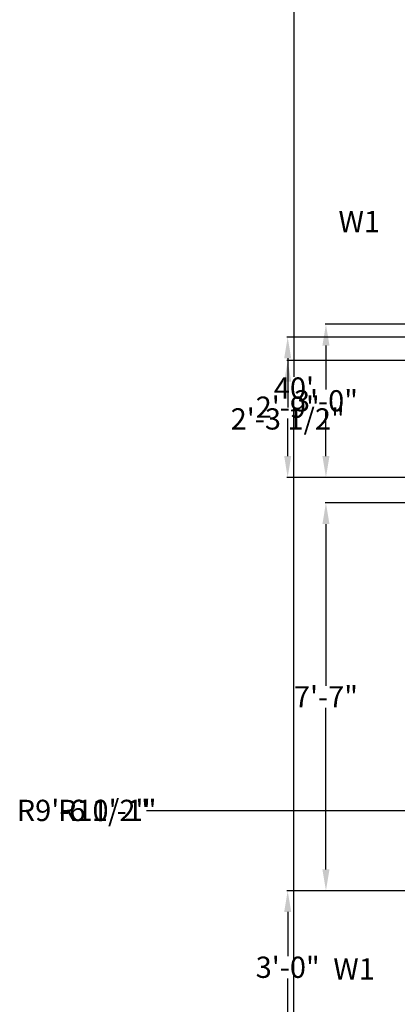
# Model space of a CAD drawing. Units: inches. Extents: x 3136 to 3620, y 13606 to 14152.
# Tile 2 of 6: x 3136 to 3225, y 13734 to 13965. Entities that reach past the tile are written whole.
import ezdxf

# ---------------------------------------------------------------- set-up
doc = ezdxf.new("R2010")
doc.units = ezdxf.units.IN
doc.layers.add('A-ANNO-DIMS', color=2, linetype='Continuous', lineweight=18)
doc.layers.add('A-ANNO-TEXT', color=7, linetype='Continuous', lineweight=18)
doc.styles.get("Standard").update_dxf_attribs({"font": 'arial.ttf', "height": 5})
doc.dimstyles.get("Standard").update_dxf_attribs({"dimtxt": 5, "dimasz": 5, "dimexe": 0.18, "dimexo": 0.0625, "dimgap": 0.09, "dimtad": 0, "dimtih": 1, "dimtoh": 1, "dimdec": 0, "dimzin": 0, "dimdsep": 46, "dimlunit": 3, "dimtxsty": 'Standard', "dimcen": 0.09, "dimadec": 0, "dimazin": 0, "dimtfac": 1, "dimtdec": 0, "dimtofl": 0, "dimtmove": 0, "dimatfit": 3, "dimfxl": 1, "dimtolj": 1, "dimtzin": 0, "dimarcsym": 0})

# ---------------------------------------------------------------- blocks, each defined once
blk = doc.blocks.new('*D28')
at = {"layer": 'A-ANNO-DIMS', "color": 0, "lineweight": -2, "transparency": 16777216}
for p, q in [((3224.81, 14118.84), (3200.37, 14118.84)), ((3200.55, 14113.84), (3200.55, 13881.48)), ((3200.55, 13643.84), (3200.55, 13876.2)), ((3224.81, 13638.84), (3200.37, 13638.84))]:
    blk.add_line(p, q, dxfattribs=at)
at = {"layer": 'A-ANNO-DIMS', "color": 0, "transparency": 16777216}
for points in [[(3199.71, 14113.84), (3201.38, 14113.84), (3200.55, 14118.84)], [(3199.71, 13643.84), (3201.38, 13643.84), (3200.55, 13638.84)]]:
    blk.add_solid(points, dxfattribs=at)
at = {"layer": 'Defpoints', "color": 0, "transparency": 16777216}
for p in [(3200.55, 14118.84), (3224.87, 14118.84), (3224.87, 13638.84)]:
    blk.add_point(p, dxfattribs=at)
at = {"layer": 'A-ANNO-DIMS', "color": 0, "transparency": 16777216, "insert": (3200.55, 13878.84), "char_height": 5, "attachment_point": 5}
blk.add_mtext("\\A1;40'", dxfattribs=at)
blk = doc.blocks.new('*D49')
at = {"layer": 'A-ANNO-DIMS', "color": 0, "lineweight": -2, "transparency": 16777216}
for p, q in [((3503.81, 13885.32), (3198.89, 13885.32)), ((3199.07, 13880.32), (3199.07, 13874.26)), ((3199.07, 13862.84), (3199.07, 13868.9)), ((3503.81, 13857.84), (3198.89, 13857.84))]:
    blk.add_line(p, q, dxfattribs=at)
at = {"layer": 'A-ANNO-DIMS', "color": 0, "transparency": 16777216}
for points in [[(3198.24, 13880.32), (3199.9, 13880.32), (3199.07, 13885.32)], [(3198.24, 13862.84), (3199.9, 13862.84), (3199.07, 13857.84)]]:
    blk.add_solid(points, dxfattribs=at)
at = {"layer": 'Defpoints', "color": 0, "transparency": 16777216}
for p in [(3199.07, 13885.32), (3503.87, 13885.32), (3503.87, 13857.84)]:
    blk.add_point(p, dxfattribs=at)
at = {"layer": 'A-ANNO-DIMS', "color": 0, "transparency": 16777216, "insert": (3199.07, 13871.58), "char_height": 5, "attachment_point": 5}
blk.add_mtext('\\A1;2\'-3 1/2"', dxfattribs=at)
blk = doc.blocks.new('*D51')
at = {"layer": 'A-ANNO-DIMS', "color": 0, "lineweight": -2, "transparency": 16777216}
for p, q in [((3224.81, 13760.63), (3198.89, 13760.63)), ((3199.07, 13755.63), (3199.07, 13745.27)), ((3199.07, 13729.63), (3199.07, 13739.99)), ((3224.81, 13724.63), (3198.89, 13724.63))]:
    blk.add_line(p, q, dxfattribs=at)
at = {"layer": 'A-ANNO-DIMS', "color": 0, "transparency": 16777216}
for points in [[(3198.24, 13755.63), (3199.9, 13755.63), (3199.07, 13760.63)], [(3198.24, 13729.63), (3199.9, 13729.63), (3199.07, 13724.63)]]:
    blk.add_solid(points, dxfattribs=at)
at = {"layer": 'Defpoints', "color": 0, "transparency": 16777216}
for p in [(3199.07, 13760.63), (3224.87, 13760.63), (3224.87, 13724.63)]:
    blk.add_point(p, dxfattribs=at)
at = {"layer": 'A-ANNO-DIMS', "color": 0, "transparency": 16777216, "insert": (3199.07, 13742.63), "char_height": 5, "attachment_point": 5}
blk.add_mtext('\\A1;3\'-0"', dxfattribs=at)
blk = doc.blocks.new('*D63')
at = {"layer": 'A-ANNO-DIMS', "color": 0, "lineweight": -2, "transparency": 16777216}
for p, q in [((3233.81, 13851.84), (3207.89, 13851.84)), ((3208.07, 13846.84), (3208.07, 13808.82)), ((3208.07, 13765.63), (3208.07, 13803.64)), ((3233.81, 13760.63), (3207.89, 13760.63))]:
    blk.add_line(p, q, dxfattribs=at)
at = {"layer": 'A-ANNO-DIMS', "color": 0, "transparency": 16777216}
for points in [[(3207.24, 13846.84), (3208.9, 13846.84), (3208.07, 13851.84)], [(3207.24, 13765.63), (3208.9, 13765.63), (3208.07, 13760.63)]]:
    blk.add_solid(points, dxfattribs=at)
at = {"layer": 'Defpoints', "color": 0, "transparency": 16777216}
for p in [(3208.07, 13851.84), (3233.87, 13851.84), (3233.87, 13760.63)]:
    blk.add_point(p, dxfattribs=at)
at = {"layer": 'A-ANNO-DIMS', "color": 0, "transparency": 16777216, "insert": (3208.07, 13806.23), "char_height": 5, "attachment_point": 5}
blk.add_mtext('\\A1;7\'-7"', dxfattribs=at)
blk = doc.blocks.new('*D64')
at = {"layer": 'A-ANNO-DIMS', "color": 0, "lineweight": -2, "transparency": 16777216}
for p, q in [((3233.81, 13893.84), (3207.89, 13893.84)), ((3208.07, 13888.84), (3208.07, 13878.48)), ((3208.07, 13862.84), (3208.07, 13873.19)), ((3233.81, 13857.84), (3207.89, 13857.84))]:
    blk.add_line(p, q, dxfattribs=at)
at = {"layer": 'A-ANNO-DIMS', "color": 0, "transparency": 16777216}
for points in [[(3207.24, 13888.84), (3208.9, 13888.84), (3208.07, 13893.84)], [(3207.24, 13862.84), (3208.9, 13862.84), (3208.07, 13857.84)]]:
    blk.add_solid(points, dxfattribs=at)
at = {"layer": 'Defpoints', "color": 0, "transparency": 16777216}
for p in [(3208.07, 13893.84), (3233.87, 13893.84), (3233.87, 13857.84)]:
    blk.add_point(p, dxfattribs=at)
at = {"layer": 'A-ANNO-DIMS', "color": 0, "transparency": 16777216, "insert": (3208.07, 13875.84), "char_height": 5, "attachment_point": 5}
blk.add_mtext('\\A1;3\'-0"', dxfattribs=at)
blk = doc.blocks.new('*D73')
at = {"layer": 'A-ANNO-DIMS', "color": 0, "lineweight": -2, "transparency": 16777216}
for p, q in [((3551.42, 13890.84), (3198.89, 13890.84)), ((3199.07, 13885.84), (3199.07, 13876.98)), ((3199.07, 13862.84), (3199.07, 13871.7)), ((3540.92, 13857.84), (3198.89, 13857.84))]:
    blk.add_line(p, q, dxfattribs=at)
at = {"layer": 'A-ANNO-DIMS', "color": 0, "transparency": 16777216}
for points in [[(3198.24, 13885.84), (3199.9, 13885.84), (3199.07, 13890.84)], [(3198.24, 13862.84), (3199.9, 13862.84), (3199.07, 13857.84)]]:
    blk.add_solid(points, dxfattribs=at)
at = {"layer": 'Defpoints', "color": 0, "transparency": 16777216}
for p in [(3551.48, 13890.84), (3199.07, 13857.84), (3540.98, 13857.84)]:
    blk.add_point(p, dxfattribs=at)
at = {"layer": 'A-ANNO-DIMS', "color": 0, "transparency": 16777216, "insert": (3199.07, 13874.34), "char_height": 5, "attachment_point": 5}
blk.add_mtext('\\A1;2\'-9"', dxfattribs=at)
blk = doc.blocks.new('*D78')
at = {"layer": 'A-ANNO-DIMS', "color": 0, "lineweight": -2, "transparency": 16777216}
for p, q in [((3167.68, 13779.52), (3235.4, 13779.52)), ((3361.5, 13779.52), (3361.68, 13779.52)), ((3361.59, 13779.43), (3361.59, 13779.61))]:
    blk.add_line(p, q, dxfattribs=at)
at = {"layer": 'A-ANNO-DIMS', "color": 0, "transparency": 16777216}
blk.add_solid([(3235.4, 13780.35), (3235.4, 13778.68), (3240.4, 13779.52)], dxfattribs=at)
at = {"layer": 'Defpoints', "color": 0, "transparency": 16777216}
for p in [(3240.4, 13779.52), (3361.59, 13779.52)]:
    blk.add_point(p, dxfattribs=at)
at = {"layer": 'A-ANNO-DIMS', "color": 0, "transparency": 16777216, "insert": (3156.61, 13779.52), "char_height": 5, "attachment_point": 5}
blk.add_mtext('\\A1;R10\'-1"', dxfattribs=at)
blk = doc.blocks.new('*D79')
at = {"layer": 'A-ANNO-DIMS', "color": 0, "lineweight": -2, "transparency": 16777216}
for p, q in [((3165.85, 13779.52), (3229.4, 13779.52)), ((3348.56, 13779.52), (3348.74, 13779.52)), ((3348.65, 13779.43), (3348.65, 13779.61))]:
    blk.add_line(p, q, dxfattribs=at)
at = {"layer": 'A-ANNO-DIMS', "color": 0, "transparency": 16777216}
blk.add_solid([(3229.4, 13780.35), (3229.4, 13778.68), (3234.4, 13779.52)], dxfattribs=at)
at = {"layer": 'Defpoints', "color": 0, "transparency": 16777216}
for p in [(3234.4, 13779.52), (3348.65, 13779.52)]:
    blk.add_point(p, dxfattribs=at)
at = {"layer": 'A-ANNO-DIMS', "color": 0, "transparency": 16777216, "insert": (3150.89, 13779.52), "char_height": 5, "attachment_point": 5}
blk.add_mtext('\\A1;R9\'-6 1/2"', dxfattribs=at)

msp = doc.modelspace()

# ---------------------------------------------------------------- texts
at = {"layer": 'A-ANNO-TEXT', "char_height": 5, "attachment_point": 1}
for insert in [(3204.78, 13920.49), (3203.56, 13744.75)]:
    msp.add_mtext_dynamic_manual_height_columns('\\pxqc;W1', width=22.2613, gutter_width=25, heights=[0], dxfattribs=dict(at, insert=insert))

# ---------------------------------------------------------------- dimensions: what is measured, and where the dimension line sits
at = {"layer": 'A-ANNO-DIMS'}
for base, p1, p2, override, picture, middle in [((3200.55, 14118.84), (3224.87, 13638.84), (3224.87, 14118.84), {"dimclrd": 0, "dimclre": 0, "dimclrt": 0}, '*D28', (3200.55, 13878.84)), ((3208.07, 13893.84), (3233.87, 13857.84), (3233.87, 13893.84), {"dimdec": 1, "dimlfac": 1, "dimrnd": 0, "dimzin": 1, "dimdsep": 46, "dimlunit": 4, "dimfrac": 2}, '*D64', (3208.07, 13875.84)), ((3199.07, 13857.84), (3551.48, 13890.84), (3540.98, 13857.84), {"dimdec": 1, "dimlfac": 1, "dimrnd": 0, "dimzin": 1, "dimdsep": 46, "dimlunit": 4, "dimfrac": 2}, '*D73', (3199.07, 13874.34)), ((3199.07, 13885.32), (3503.87, 13857.84), (3503.87, 13885.32), {"dimdec": 1, "dimlfac": 1, "dimrnd": 0, "dimzin": 1, "dimdsep": 46, "dimlunit": 4, "dimfrac": 2}, '*D49', (3199.07, 13871.58)), ((3208.07, 13851.84), (3233.87, 13760.63), (3233.87, 13851.84), {"dimdec": 1, "dimlfac": 1, "dimrnd": 0, "dimzin": 1, "dimdsep": 46, "dimlunit": 4, "dimfrac": 2}, '*D63', (3208.07, 13806.23)), ((3199.07, 13760.63), (3224.87, 13724.63), (3224.87, 13760.63), {"dimdec": 1, "dimlfac": 1, "dimrnd": 0, "dimzin": 1, "dimdsep": 46, "dimlunit": 4, "dimfrac": 2}, '*D51', (3199.07, 13742.63))]:
    dim = msp.add_linear_dim(base=base, p1=p1, p2=p2, angle=90, dimstyle='Standard', override=override, dxfattribs=at)
    dim.commit()
    dim.dimension.update_dxf_attribs({"geometry": picture, "text_midpoint": middle})
for center, mpoint, picture, middle in [((3348.64777, 13779.517148), (3234.39777, 13779.517), '*D79', (3165.84777, 13779.5169112)), ((3361.59, 13779.52), (3240.4, 13779.52), '*D78', (3167.68, 13779.52))]:
    dim = msp.add_radius_dim(center=center, mpoint=mpoint, dimstyle='Standard', override={"dimdec": 1, "dimlfac": 1, "dimrnd": 0, "dimzin": 1, "dimdsep": 46, "dimlunit": 4, "dimfrac": 2}, dxfattribs=at)
    dim.commit()
    dim.dimension.update_dxf_attribs({"geometry": picture, "text_midpoint": middle, "dimtype": 164})

doc.saveas('drawing.dxf')
